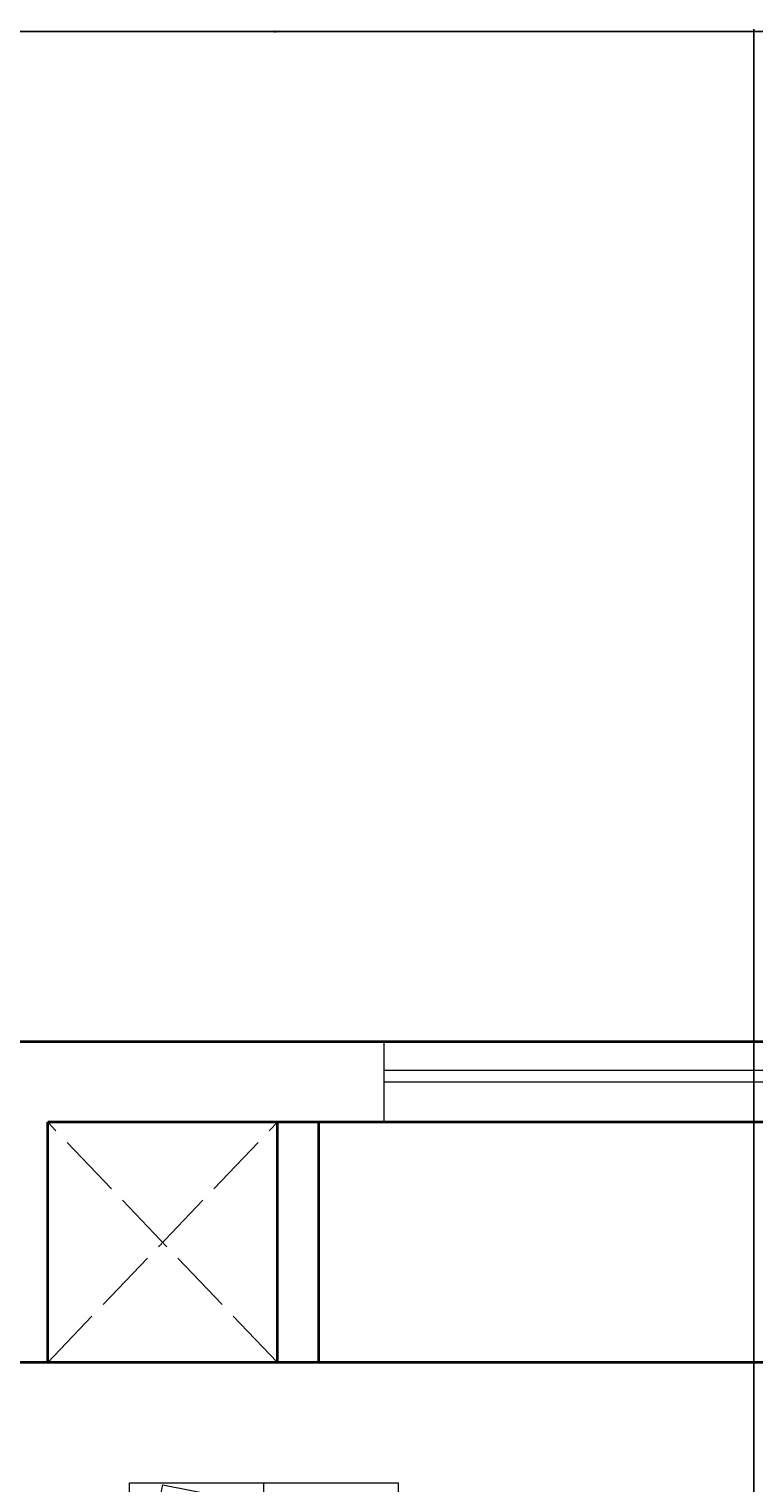
# Model space of a CAD drawing. Units: inches. Extents: x -61 to 1599, y -1316 to 257.
# Tile 143 of 204: x 294 to 348, y 149 to 257. Entities that reach past the tile are written whole.
import ezdxf

# ---------------------------------------------------------------- set-up
doc = ezdxf.new("R2010")
doc.units = ezdxf.units.IN
doc.header["$MEASUREMENT"] = 0
doc.linetypes.add('ACAD_ISO02W100', pattern=[15, 12, -3])
for name, color, linetype, lineweight in [('A-ANNO-DIMS', 2, 'Continuous', 18), ('A-FLOR-CASE', 8, 'Continuous', 18), ('A-FLOR-OPEN-HIDN', 8, 'ACAD_ISO02W100', 13), ('WALLS', 4, 'Continuous', 35), ('WINDOWS', 220, 'Continuous', 18)]:
    doc.layers.add(name, color=color, linetype=linetype, lineweight=lineweight)
doc.styles.get("Standard").update_dxf_attribs({"font": 'arial.ttf'})
doc.dimstyles.get("Standard").update_dxf_attribs({"dimtxt": 0.18, "dimasz": 0.18, "dimexe": 0.18, "dimexo": 0.0625, "dimgap": 0.09, "dimtad": 0, "dimtih": 1, "dimtoh": 1, "dimdec": 0, "dimzin": 0, "dimdsep": 46, "dimlunit": 3, "dimtxsty": 'Standard', "dimcen": 0.09, "dimadec": 0, "dimazin": 0, "dimtfac": 1, "dimtdec": 0, "dimtofl": 0, "dimtmove": 0, "dimatfit": 3, "dimfxl": 1, "dimtolj": 1, "dimtzin": 0, "dimarcsym": 0})

# ---------------------------------------------------------------- blocks, each defined once
blk = doc.blocks.new('WIN-51IN')
for p, q in [((0, 0), (0, 6)), ((50.52, 0), (50.52, 6)), ((0, 3.89), (50.52, 3.89)), ((0, 3), (50.52, 3))]:
    blk.add_line(p, q)
blk = doc.blocks.new('WARDROBE-HANGING')
blk.add_line((10.05, 0), (10.05, 68))
for points in [[(20.09, 0), (0, 0), (0, 68), (20.09, 68)], [(2.48, 67.85), (17.75, 64.85), (17.61, 64.14), (2.34, 67.15)], [(1.35, 59.16), (16.22, 63.73), (16.43, 63.04), (1.56, 58.47)], [(1.32, 62.96), (16.59, 59.95), (16.45, 59.25), (1.19, 62.25)], [(1.71, 56.78), (16.98, 53.78), (16.84, 53.07), (1.57, 56.08)], [(1, 46.47), (15.87, 51.04), (16.08, 50.35), (1.21, 45.78)], [(1.39, 50.01), (16.66, 47.01), (16.52, 46.3), (1.26, 49.31)], [(1.36, 44.09), (16.63, 41.09), (16.49, 40.38), (1.23, 43.38)], [(1.26, 37.2), (16.53, 34.2), (16.39, 33.49), (1.12, 36.5)], [(1.28, 33.41), (16.16, 37.98), (16.37, 37.29), (1.49, 32.72)], [(1.65, 31.03), (16.92, 28.03), (16.78, 27.32), (1.51, 30.32)], [(1.26, 25.09), (16.53, 22.09), (16.39, 21.38), (1.12, 24.39)], [(1.28, 21.3), (16.15, 25.87), (16.36, 25.18), (1.49, 20.61)], [(1.65, 18.92), (16.91, 15.92), (16.78, 15.21), (1.51, 18.21)], [(1.93, 9.89), (16.8, 14.46), (17.01, 13.77), (2.14, 9.2)], [(1.91, 13.69), (17.17, 10.68), (17.04, 9.98), (1.77, 12.98)], [(2.29, 7.51), (17.56, 4.51), (17.42, 3.8), (2.16, 6.81)], [(17.49, 1.96), (1.93, 1.96), (1.93, 2.68), (17.49, 2.68)]]:
    blk.add_lwpolyline(points, close=True)
blk = doc.blocks.new('*D686')
at = {"layer": 'A-ANNO-DIMS', "color": 0, "lineweight": -2, "transparency": 16777216}
for p, q in [((14.7, 157.74), (14.7, 257.46)), ((14.88, 257.28), (768.35, 257.28)), ((1522.52, 257.28), (769.05, 257.28)), ((1522.7, 157.74), (1522.7, 257.46))]:
    blk.add_line(p, q, dxfattribs=at)
at = {"layer": 'A-ANNO-DIMS', "color": 0, "transparency": 16777216}
for points in [[(14.88, 257.31), (14.88, 257.25), (14.7, 257.28)], [(1522.52, 257.31), (1522.52, 257.25), (1522.7, 257.28)]]:
    blk.add_solid(points, dxfattribs=at)
at = {"layer": 'DEFPOINTS', "color": 0, "transparency": 16777216}
for p in [(1522.7, 257.28), (14.7, 157.68), (1522.7, 157.68)]:
    blk.add_point(p, dxfattribs=at)
at = {"layer": 'A-ANNO-DIMS', "color": 0, "transparency": 16777216, "insert": (768.7, 257.28), "char_height": 0.18, "attachment_point": 5}
blk.add_mtext('\\A1;1508', dxfattribs=at)
blk = doc.blocks.new('*D687')
at = {"layer": 'A-ANNO-DIMS', "color": 0, "lineweight": -2, "transparency": 16777216}
for p, q in [((289.42, 181.68), (-61.08, 181.68)), ((-60.9, 181.5), (-60.9, -528.95)), ((-60.9, -1239.76), (-60.9, -529.32)), ((319.64, -1239.94), (-61.08, -1239.94))]:
    blk.add_line(p, q, dxfattribs=at)
at = {"layer": 'A-ANNO-DIMS', "color": 0, "transparency": 16777216}
for points in [[(-60.93, 181.5), (-60.87, 181.5), (-60.9, 181.68)], [(-60.93, -1239.76), (-60.87, -1239.76), (-60.9, -1239.94)]]:
    blk.add_solid(points, dxfattribs=at)
at = {"layer": 'DEFPOINTS', "color": 0, "transparency": 16777216}
for p in [(289.48, 181.68), (-60.9, -1239.94), (319.7, -1239.94)]:
    blk.add_point(p, dxfattribs=at)
at = {"layer": 'A-ANNO-DIMS', "color": 0, "transparency": 16777216, "insert": (-60.9, -529.13), "char_height": 0.18, "attachment_point": 5}
blk.add_mtext('\\A1;1421.6', dxfattribs=at)
blk = doc.blocks.new('*D702')
at = {"layer": 'A-ANNO-DIMS', "color": 0, "lineweight": -2, "transparency": 16777216}
for p, q in [((276.88, -616.88), (276.88, 257.46)), ((277.06, 257.28), (312.21, 257.28)), ((348.14, 257.28), (312.99, 257.28)), ((348.32, -616.88), (348.32, 257.46))]:
    blk.add_line(p, q, dxfattribs=at)
at = {"layer": 'A-ANNO-DIMS', "color": 0, "transparency": 16777216}
for points in [[(277.06, 257.31), (277.06, 257.25), (276.88, 257.28)], [(348.14, 257.31), (348.14, 257.25), (348.32, 257.28)]]:
    blk.add_solid(points, dxfattribs=at)
at = {"layer": 'DEFPOINTS', "color": 0, "transparency": 16777216}
for p in [(348.32, 257.28), (276.88, -616.94), (348.32, -616.94)]:
    blk.add_point(p, dxfattribs=at)
at = {"layer": 'A-ANNO-DIMS', "color": 0, "transparency": 16777216, "insert": (312.6, 257.28), "char_height": 0.18, "attachment_point": 5}
blk.add_mtext('\\A1;71.44', dxfattribs=at)

msp = doc.modelspace()

# ---------------------------------------------------------------- linework, layer by layer
at = {"layer": 'A-FLOR-OPEN-HIDN', "ltscale": 0.4}
for p, q in [((295.4807, 157.6771), (312.6819, 175.6771)), ((312.6819, 157.6771), (295.4807, 175.6771))]:
    msp.add_line(p, q, dxfattribs=at)
at = {"layer": 'WALLS'}
for p, q in [((403.7028, 181.6771), (289.4807, 181.6771)), ((295.4807, 157.6771), (295.4807, 175.6771)), ((397.7028, 175.6771), (295.4807, 175.6771)), ((312.6819, 157.6771), (312.6819, 175.6771)), ((315.7747, 157.6771), (315.7747, 175.6771)), ((544.7028, 157.6771), (14.7028, 157.6771))]:
    msp.add_line(p, q, dxfattribs=at)

# ---------------------------------------------------------------- block references
at = {"layer": 'A-FLOR-CASE'}
msp.add_blockref('WARDROBE-HANGING', (301.609, 80.677), dxfattribs=at)
at = {"layer": 'WINDOWS'}
msp.add_blockref('WIN-51IN', (320.659, 175.677), dxfattribs=at)

# ---------------------------------------------------------------- dimensions: what is measured, and where the dimension line sits
at = {"layer": 'A-ANNO-DIMS'}
for base, p1, p2, override, picture, middle in [((1522.7028, 257.2771), (14.7028, 157.6771), (1522.7028, 157.6771), {"dimdec": 0, "dimlfac": 1, "dimrnd": 0, "dimzin": 0, "dimdsep": 46, "dimlunit": 2}, '*D686', (768.7028, 257.2771)), ((348.3201, 257.2771), (276.8825, -616.9446), (348.3201, -616.9446), {"dimdec": 2, "dimlfac": 1, "dimrnd": 0, "dimzin": 0, "dimdsep": 46, "dimlunit": 2}, '*D702', (312.6013, 257.2771))]:
    dim = msp.add_linear_dim(base=base, p1=p1, p2=p2, dimstyle='Standard', override=override, dxfattribs=at)
    dim.commit()
    dim.dimension.update_dxf_attribs({"geometry": picture, "text_midpoint": middle})
dim = msp.add_linear_dim(base=(-60.8972, -1239.9446), p1=(289.4807, 181.6771), p2=(319.7028, -1239.9446), angle=90, dimstyle='Standard', override={"dimdec": 1, "dimlfac": 1, "dimrnd": 0, "dimzin": 0, "dimdsep": 46, "dimlunit": 2}, dxfattribs=at)
dim.commit()
dim.dimension.update_dxf_attribs({"geometry": '*D687', "text_midpoint": (-60.8972, -529.1337)})

doc.saveas('drawing.dxf')
